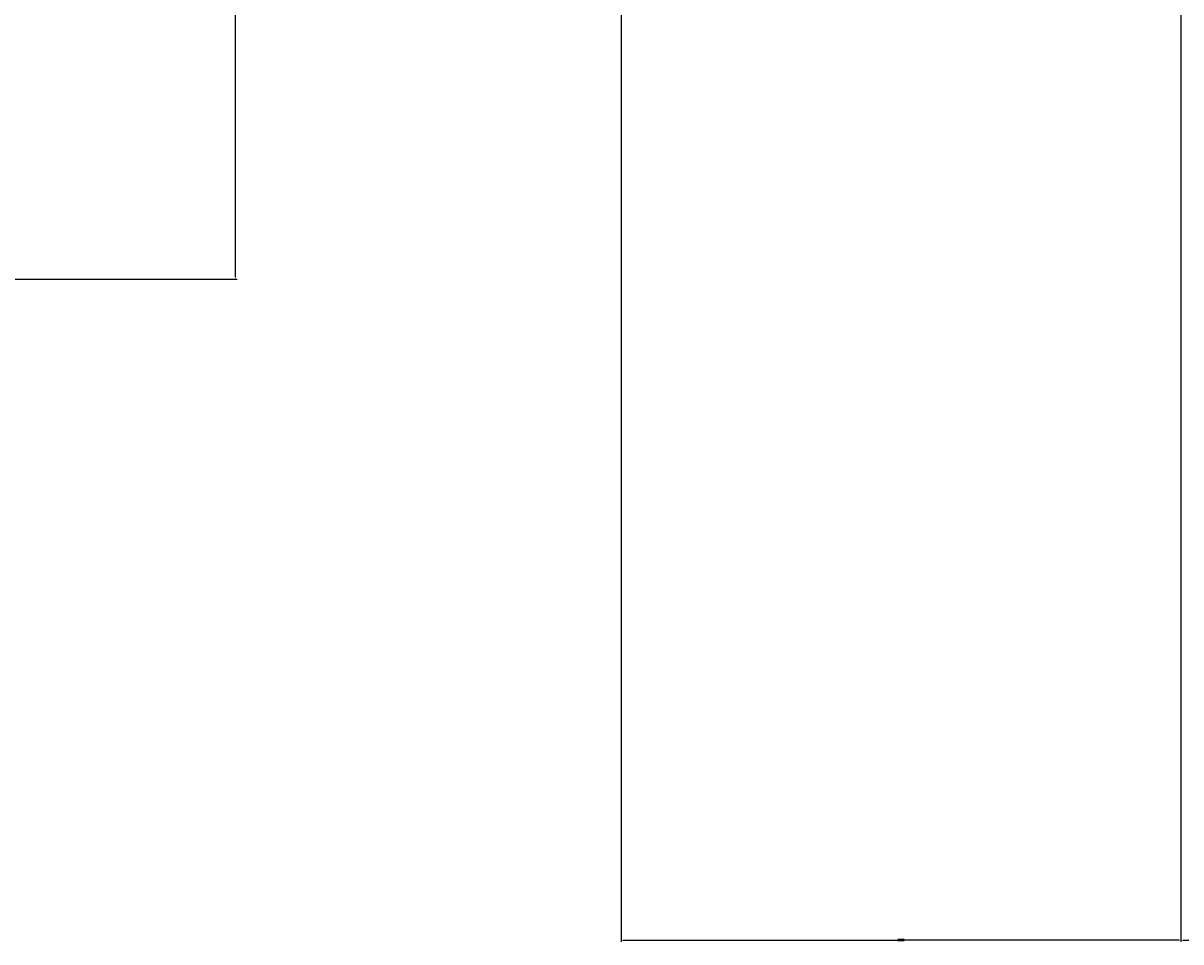
# Model space of a CAD drawing. Units: inches. Extents: x -301 to 715, y -607 to 364.
# Tile 126 of 141: x 194 to 310, y -607 to -515. Entities that reach past the tile are written whole.
import ezdxf

# ---------------------------------------------------------------- set-up
doc = ezdxf.new("R2010")
doc.units = ezdxf.units.IN
doc.header["$MEASUREMENT"] = 0
doc.layers.add('A-ANNO-DIMS', color=2, linetype='Continuous', lineweight=18)
doc.styles.get("Standard").update_dxf_attribs({"font": 'arial.ttf'})
doc.dimstyles.get("Standard").update_dxf_attribs({"dimtxt": 0.18, "dimasz": 0.18, "dimexe": 0.18, "dimexo": 0.0625, "dimgap": 0.09, "dimtad": 0, "dimtih": 1, "dimtoh": 1, "dimdec": 1, "dimzin": 0, "dimdsep": 46, "dimlunit": 4, "dimtxsty": 'Standard', "dimcen": 0.09, "dimclrd": 3, "dimclre": 4, "dimclrt": 6, "dimadec": 0, "dimazin": 0, "dimtfac": 1, "dimtdec": 1, "dimtofl": 0, "dimtmove": 0, "dimatfit": 3, "dimfxl": 1, "dimtfill": 2, "dimtfillclr": 51, "dimtolj": 1, "dimtzin": 0, "dimarcsym": 0})

# ---------------------------------------------------------------- blocks, each defined once
blk = doc.blocks.new('*D176')
at = {"layer": 'A-ANNO-DIMS', "color": 4, "lineweight": -2, "transparency": 16777216}
for p, q in [((148.28, -324.48), (215.61, -324.48)), ((-15.22, -540.48), (215.61, -540.48))]:
    blk.add_line(p, q, dxfattribs=at)
at = {"layer": 'A-ANNO-DIMS', "color": 3, "lineweight": -2, "transparency": 16777216}
for p, q in [((215.43, -324.66), (215.43, -432.3)), ((215.43, -540.3), (215.43, -432.66))]:
    blk.add_line(p, q, dxfattribs=at)
at = {"layer": 'A-ANNO-DIMS', "color": 3, "transparency": 16777216}
for points in [[(215.4, -324.66), (215.46, -324.66), (215.43, -324.48)], [(215.4, -540.3), (215.46, -540.3), (215.43, -540.48)]]:
    blk.add_solid(points, dxfattribs=at)
at = {"layer": 'Defpoints', "color": 0, "transparency": 16777216}
for p in [(148.22, -324.48), (-15.28, -540.48), (215.43, -540.48)]:
    blk.add_point(p, dxfattribs=at)
at = {"layer": 'A-ANNO-DIMS', "color": 6, "transparency": 16777216, "insert": (215.43, -432.48), "char_height": 0.18, "attachment_point": 5, "bg_fill": 1, "box_fill_scale": 1.25, "bg_fill_color": 51, "bg_fill_transparency": 0}
blk.add_mtext('\\A1;18\'-0"', dxfattribs=at)
blk = doc.blocks.new('*D194')
at = {"layer": 'A-ANNO-DIMS', "color": 4, "lineweight": -2, "transparency": 16777216}
for p, q in [((310.02, -441.61), (310.02, -606.79)), ((254.02, -507.61), (254.02, -606.79))]:
    blk.add_line(p, q, dxfattribs=at)
at = {"layer": 'A-ANNO-DIMS', "color": 3, "lineweight": -2, "transparency": 16777216}
for p, q in [((254.2, -606.61), (281.68, -606.61)), ((309.84, -606.61), (282.35, -606.61))]:
    blk.add_line(p, q, dxfattribs=at)
at = {"layer": 'A-ANNO-DIMS', "color": 3, "transparency": 16777216}
for points in [[(254.2, -606.58), (254.2, -606.64), (254.02, -606.61)], [(309.84, -606.58), (309.84, -606.64), (310.02, -606.61)]]:
    blk.add_solid(points, dxfattribs=at)
at = {"layer": 'Defpoints', "color": 0, "transparency": 16777216}
for p in [(310.02, -441.55), (254.02, -507.55), (310.02, -606.61)]:
    blk.add_point(p, dxfattribs=at)
at = {"layer": 'A-ANNO-DIMS', "color": 6, "transparency": 16777216, "insert": (282.02, -606.61), "char_height": 0.18, "attachment_point": 5, "bg_fill": 1, "box_fill_scale": 1.25, "bg_fill_color": 51, "bg_fill_transparency": 0}
blk.add_mtext('\\A1;4\'-8"', dxfattribs=at)
blk = doc.blocks.new('*D195')
at = {"layer": 'A-ANNO-DIMS', "color": 4, "lineweight": -2, "transparency": 16777216}
for p, q in [((310.02, -441.61), (310.02, -606.79)), ((360.02, -441.61), (360.02, -606.79))]:
    blk.add_line(p, q, dxfattribs=at)
at = {"layer": 'A-ANNO-DIMS', "color": 3, "lineweight": -2, "transparency": 16777216}
for p, q in [((310.2, -606.61), (334.68, -606.61)), ((359.84, -606.61), (335.35, -606.61))]:
    blk.add_line(p, q, dxfattribs=at)
at = {"layer": 'A-ANNO-DIMS', "color": 3, "transparency": 16777216}
for points in [[(310.2, -606.58), (310.2, -606.64), (310.02, -606.61)], [(359.84, -606.58), (359.84, -606.64), (360.02, -606.61)]]:
    blk.add_solid(points, dxfattribs=at)
at = {"layer": 'Defpoints', "color": 0, "transparency": 16777216}
for p in [(310.02, -441.55), (360.02, -441.55), (360.02, -606.61)]:
    blk.add_point(p, dxfattribs=at)
at = {"layer": 'A-ANNO-DIMS', "color": 6, "transparency": 16777216, "insert": (335.02, -606.61), "char_height": 0.18, "attachment_point": 5, "bg_fill": 1, "box_fill_scale": 1.25, "bg_fill_color": 51, "bg_fill_transparency": 0}
blk.add_mtext('\\A1;4\'-2"', dxfattribs=at)

msp = doc.modelspace()

# ---------------------------------------------------------------- dimensions: what is measured, and where the dimension line sits
at = {"layer": 'A-ANNO-DIMS'}
dim = msp.add_linear_dim(base=(215.43, -540.48), p1=(148.22, -324.48), p2=(-15.28, -540.48), angle=90, dimstyle='Standard', override={"dimdec": 1, "dimlfac": 1, "dimrnd": 0, "dimzin": 1, "dimdsep": 46, "dimlunit": 4, "dimfrac": 2}, dxfattribs=at)
dim.commit()
dim.dimension.update_dxf_attribs({"geometry": '*D176', "text_midpoint": (215.43, -432.48)})
for base, p1, p2, picture, middle in [((310.02, -606.61), (254.02, -507.55), (310.02, -441.55), '*D194', (282.02, -606.61)), ((360.02, -606.61), (310.02, -441.55), (360.02, -441.55), '*D195', (335.02, -606.61))]:
    dim = msp.add_linear_dim(base=base, p1=p1, p2=p2, dimstyle='Standard', override={"dimdec": 1, "dimlfac": 1, "dimrnd": 0, "dimzin": 1, "dimdsep": 46, "dimlunit": 4, "dimfrac": 2}, dxfattribs=at)
    dim.commit()
    dim.dimension.update_dxf_attribs({"geometry": picture, "text_midpoint": middle})

doc.saveas('drawing.dxf')
